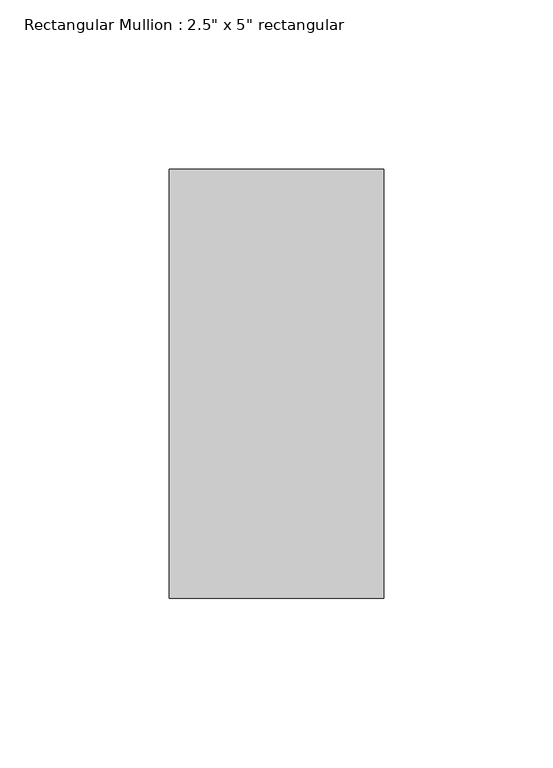
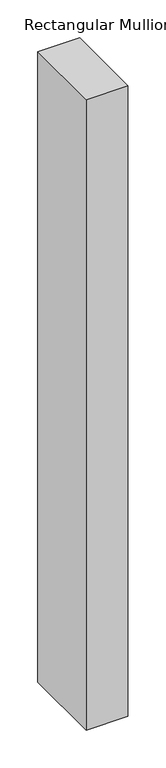
"""IFC4 building model written with IfcOpenShell, lengths in millimetres: member geometry."""

from ifc_helpers import new_model, si_unit, frame, origin, place, context, project, spatial, polyline, outline, extrude, source, transform, mapped, element, save


def member_7d21ba3d(model_context):
    return source(origin(), model_context, "Body", "SweptSolid", [
        extrude(outline(polyline([(0.0, 63.5), (0.0, -63.5), (-63.5, -63.5), (-63.5, 63.5), (0.0, 63.5)])), frame((0.0, 0.0, -1013.8675922), z_axis=(0.0, 0.0, 1.0), x_axis=(1.0, 0.0, 0.0)), (0.0, 0.0, 1.0), 1013.8675922),
    ])


if __name__ == "__main__":
    model = new_model("IFC4")
    model_context = context("Model", 3, world=origin())
    ifc_project = project(units=[si_unit("LENGTHUNIT", "METRE", prefix="MILLI")], contexts=[model_context])
    site = spatial("IfcSite", under=ifc_project)
    building = spatial("IfcBuilding", under=site)
    placement = place(None, origin())
    member_shape = member_7d21ba3d(model_context)
    element("IfcMember", 1, ObjectType="Rectangular Mullion : 2.5\" x 5\" rectangular", at=placement, inside=building, context=model_context, shape_type="MappedRepresentation", body=[
        mapped(member_shape, transform((0.0, 0.0, 0.0), x_axis=(1.0, 0.0, 0.0), y_axis=(0.0, 1.0, 0.0), z_axis=(0.0, 0.0, 1.0))),
    ])
    save(model, "model.ifc")

# Revit data of these elements
# Type "Rectangular Mullion : 2.5\" x 5\" rectangular"
#   built-in parameter 1007304 = 0.416667 (stored number, unit not read)
#   built-in parameter 1007301 = 0.104167 (stored number, unit not read)
#   built-in parameter 1007300 = 0.104167 (stored number, unit not read)
# Element 1 (IfcMember, "Rectangular Mullion : 2.5\" x 5\" rectangular")
#   Materials on its faces: "Aluminum"
# Materials
#   "Aluminum": class "Metal", colour RGB 247 247 247, transparency 0, Description = "Aluminum 6061", Cost = 0
